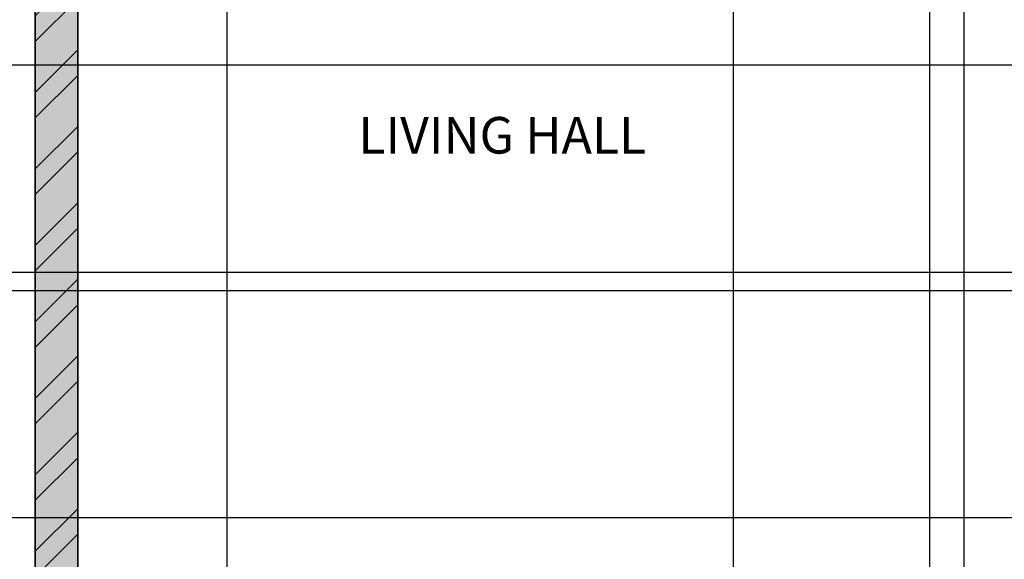
# Model space of a CAD drawing. Units: inches. Extents: x 1804 to 3296, y 909 to 2477.
# Tile 4 of 31: x 1922 to 2130, y 1215 to 1329. Entities that reach past the tile are written whole.
import ezdxf

# ---------------------------------------------------------------- set-up
doc = ezdxf.new("R2010")
doc.units = ezdxf.units.IN
for name, color, linetype, lineweight in [('A-ANNO-DIMS', 2, 'Continuous', 18), ('A-ANNO-TTLB', 156, 'Continuous', 35), ('A-AREA-IDEN', 190, 'Continuous', 18), ('A-WALL-PATT', 10, 'Continuous', 13), ('WALL', 10, 'Continuous', 35)]:
    doc.layers.add(name, color=color, linetype=linetype, lineweight=lineweight)
doc.styles.get("Standard").update_dxf_attribs({"font": 'arial.ttf'})
doc.dimstyles.new('ISO-25', dxfattribs={"dimtxt": 5, "dimasz": 2.5, "dimexe": 1.25, "dimexo": 0.625, "dimtad": 1, "dimdec": 0, "dimlunit": 4, "dimtxsty": 'Standard', "dimcen": 2.5, "dimadec": 0, "dimazin": 0, "dimtfac": 1, "dimtdec": 0, "dimtmove": 0, "dimatfit": 3, "dimfxl": 1, "dimarcsym": 0})

# ---------------------------------------------------------------- blocks, each defined once
blk = doc.blocks.new('*D21')
at = {"layer": 'A-ANNO-DIMS', "color": 0, "lineweight": -2, "transparency": 16777216}
for p, q in [((1935.21, 1539.88), (1967.44, 1539.88)), ((1966.19, 1149.57), (1966.19, 1537.38)), ((1935.21, 1147.07), (1967.44, 1147.07))]:
    blk.add_line(p, q, dxfattribs=at)
at = {"layer": 'A-ANNO-DIMS', "color": 0, "lineweight": 100, "transparency": 16777216}
for points in [[(1965.78, 1537.38), (1966.61, 1537.38), (1966.19, 1539.88)], [(1965.78, 1149.57), (1966.61, 1149.57), (1966.19, 1147.07)]]:
    blk.add_solid(points, dxfattribs=at)
at = {"layer": 'Defpoints', "color": 0, "lineweight": 100, "transparency": 16777216}
for p in [(1934.58, 1539.88), (1966.19, 1539.88), (1934.58, 1147.07)]:
    blk.add_point(p, dxfattribs=at)
at = {"layer": 'A-ANNO-DIMS', "color": 0, "transparency": 16777216, "insert": (1963.01, 1343.47), "char_height": 5, "attachment_point": 5, "rotation": 90}
blk.add_mtext('32\'-9"', dxfattribs=at)
blk = doc.blocks.new('*D52')
at = {"layer": 'A-ANNO-DIMS', "color": 0, "lineweight": -2, "transparency": 16777216}
for p, q in [((1924.96, 1830.04), (1880.63, 1830.04)), ((1881.88, 1065.27), (1881.88, 1827.54)), ((1924.96, 1062.77), (1880.63, 1062.77))]:
    blk.add_line(p, q, dxfattribs=at)
at = {"layer": 'A-ANNO-DIMS', "color": 0, "lineweight": 100, "transparency": 16777216}
for points in [[(1881.47, 1827.54), (1882.3, 1827.54), (1881.88, 1830.04)], [(1881.47, 1065.27), (1882.3, 1065.27), (1881.88, 1062.77)]]:
    blk.add_solid(points, dxfattribs=at)
at = {"layer": 'Defpoints', "color": 0, "lineweight": 100, "transparency": 16777216}
for p in [(1881.88, 1830.04), (1925.58, 1830.04), (1925.58, 1062.77)]:
    blk.add_point(p, dxfattribs=at)
at = {"layer": 'A-ANNO-DIMS', "color": 0, "transparency": 16777216, "insert": (1878.67, 1446.4), "char_height": 5, "attachment_point": 5, "rotation": 90}
blk.add_mtext('63\'-11 1/2"', dxfattribs=at)
blk = doc.blocks.new('*D59')
at = {"layer": 'A-ANNO-DIMS', "color": 0, "lineweight": -2, "transparency": 16777216}
for p, q in [((2121.83, 1590.3), (2121.83, 975.89)), ((2161.83, 1590.3), (2161.83, 975.89)), ((2124.33, 977.14), (2159.33, 977.14))]:
    blk.add_line(p, q, dxfattribs=at)
at = {"layer": 'A-ANNO-DIMS', "color": 0, "lineweight": 100, "transparency": 16777216}
for points in [[(2124.33, 977.56), (2124.33, 976.72), (2121.83, 977.14)], [(2159.33, 977.56), (2159.33, 976.72), (2161.83, 977.14)]]:
    blk.add_solid(points, dxfattribs=at)
at = {"layer": 'Defpoints', "color": 0, "lineweight": 100, "transparency": 16777216}
for p in [(2121.83, 1590.92), (2161.83, 1590.92), (2161.83, 977.14)]:
    blk.add_point(p, dxfattribs=at)
at = {"layer": 'A-ANNO-DIMS', "color": 0, "transparency": 16777216, "insert": (2141.83, 980.32), "char_height": 5, "attachment_point": 5}
blk.add_mtext('3\'-4"', dxfattribs=at)
blk = doc.blocks.new('*D60')
at = {"layer": 'A-ANNO-DIMS', "color": 0, "lineweight": -2, "transparency": 16777216}
for p, q in [((2073.08, 1544.95), (2073.08, 975.89)), ((2114.58, 1543.75), (2114.58, 975.89)), ((2112.08, 977.14), (2075.58, 977.14))]:
    blk.add_line(p, q, dxfattribs=at)
at = {"layer": 'A-ANNO-DIMS', "color": 0, "lineweight": 100, "transparency": 16777216}
for points in [[(2075.58, 977.56), (2075.58, 976.72), (2073.08, 977.14)], [(2112.08, 977.56), (2112.08, 976.72), (2114.58, 977.14)]]:
    blk.add_solid(points, dxfattribs=at)
at = {"layer": 'Defpoints', "color": 0, "lineweight": 100, "transparency": 16777216}
for p in [(2073.08, 1545.58), (2114.58, 1544.38), (2073.08, 977.14)]:
    blk.add_point(p, dxfattribs=at)
at = {"layer": 'A-ANNO-DIMS', "color": 0, "transparency": 16777216, "insert": (2093.83, 980.35), "char_height": 5, "attachment_point": 5}
blk.add_mtext('3\'-5 1/2"', dxfattribs=at)
blk = doc.blocks.new('*D63')
at = {"layer": 'A-ANNO-DIMS', "color": 0, "lineweight": -2, "transparency": 16777216}
for p, q in [((2157.95, 1319.33), (1880.63, 1319.33)), ((1881.88, 1277.99), (1881.88, 1316.83)), ((2157.95, 1275.49), (1880.63, 1275.49))]:
    blk.add_line(p, q, dxfattribs=at)
at = {"layer": 'A-ANNO-DIMS', "color": 0, "lineweight": 100, "transparency": 16777216}
for points in [[(1881.47, 1316.83), (1882.3, 1316.83), (1881.88, 1319.33)], [(1881.47, 1277.99), (1882.3, 1277.99), (1881.88, 1275.49)]]:
    blk.add_solid(points, dxfattribs=at)
at = {"layer": 'Defpoints', "color": 0, "lineweight": 100, "transparency": 16777216}
for p in [(1881.88, 1319.33), (2158.58, 1319.33), (2158.58, 1275.49)]:
    blk.add_point(p, dxfattribs=at)
at = {"layer": 'A-ANNO-DIMS', "color": 0, "transparency": 16777216, "insert": (1878.7, 1297.41), "char_height": 5, "attachment_point": 5, "rotation": 90}
blk.add_mtext('3\'-8"', dxfattribs=at)
blk = doc.blocks.new('*D70')
at = {"layer": 'A-ANNO-DIMS', "color": 0, "lineweight": -2, "transparency": 16777216}
for p, q in [((2208.56, 1271.63), (1880.63, 1271.63)), ((1881.88, 1226.13), (1881.88, 1269.13)), ((2208.56, 1223.63), (1880.63, 1223.63))]:
    blk.add_line(p, q, dxfattribs=at)
at = {"layer": 'A-ANNO-DIMS', "color": 0, "lineweight": 100, "transparency": 16777216}
for points in [[(1881.47, 1269.13), (1882.3, 1269.13), (1881.88, 1271.63)], [(1881.47, 1226.13), (1882.3, 1226.13), (1881.88, 1223.63)]]:
    blk.add_solid(points, dxfattribs=at)
at = {"layer": 'Defpoints', "color": 0, "lineweight": 100, "transparency": 16777216}
for p in [(1881.88, 1271.63), (2209.19, 1271.63), (2209.19, 1223.63)]:
    blk.add_point(p, dxfattribs=at)
at = {"layer": 'A-ANNO-DIMS', "color": 0, "transparency": 16777216, "insert": (1878.7, 1247.63), "char_height": 5, "attachment_point": 5, "rotation": 90}
blk.add_mtext('4\'-0"', dxfattribs=at)

msp = doc.modelspace()

# ---------------------------------------------------------------- hatches: boundary and pattern name
at = {"layer": 'A-ANNO-TTLB'}
h = msp.add_hatch(color=256, dxfattribs=at)
h.dxf.hatch_style = 1
h.paths.add_polyline_path([(3294.53, 2476.54), (1803.79, 2476.54), (1805.43, 909.47), (3296.17, 909.47)])
h.paths.add_polyline_path([(1811, 914.33), (1812.79, 2467.54), (3285.53, 2467.54), (3283.74, 914.33)], flags=16)
h.paths.add_polyline_path([(1925.58, 1062.77), (1925.58, 1138.07), (1925.58, 1539.88), (1925.58, 1793.38), (1925.58, 1830.04), (2325.54, 1830.04), (2325.54, 1793.38), (2325.54, 1586.42), (2325.54, 1138.07), (2325.54, 1062.77)], flags=0)
h.paths.add_polyline_path([(1997.22, 1029.4), (2008.85, 1037.96), (2008.85, 1020.84)], flags=0)
h.paths.add_polyline_path([(1934.58, 1138.07), (1934.58, 1147.07), (2078.77, 1147.07), (2078.77, 1138.07), (2060.94, 1138.07)], flags=0)
h.paths.add_polyline_path([(1944.35, 1138.07), (1944.35, 1147.07), (2056.05, 1147.07), (2056.05, 1138.07)], flags=0)
h.paths.add_polyline_path([(2222.24, 1037.96), (2233.87, 1029.4), (2222.24, 1020.84)], flags=0)
h.paths.add_polyline_path([(2061.94, 1139.07), (2061.94, 1146.07), (2077.77, 1146.07), (2077.77, 1139.07)], flags=0)
h.paths.add_polyline_path([(2149.58, 1138.07), (2149.58, 1269.44), (2158.58, 1269.44), (2158.58, 1326.69), (2149.58, 1326.69), (2149.58, 1340.94), (2139.6, 1340.94), (2139.6, 1434.25), (2149.58, 1434.25), (2149.58, 1447.36), (2158.58, 1447.36), (2158.58, 1423.87), (2158.58, 1408.06), (2198.46, 1408.06), (2198.46, 1412.56), (2282.65, 1412.56), (2282.65, 1465.94), (2316.54, 1465.94), (2316.54, 1590.92), (2192.86, 1590.92), (2192.86, 1595.3), (2291.17, 1595.3), (2291.17, 1590.92), (2316.54, 1590.92), (2316.54, 1784.38), (2300.24, 1784.38), (2300.24, 1757.47), (2268, 1757.47), (2268, 1681.04), (2180.87, 1681.04), (2180.87, 1757.47), (2148.63, 1757.47), (2148.63, 1784.38), (2119.08, 1784.38), (2119.08, 1585.58), (2114.58, 1585.58), (2114.58, 1784.38), (2064.11, 1784.38), (2046.28, 1784.38), (2046.28, 1760.38), (1958.58, 1760.38), (1958.58, 1664.38), (1934.58, 1664.38), (1934.58, 1784.38), (1934.58, 1793.38), (2046.28, 1793.38), (2064.11, 1793.38), (2119.08, 1793.38), (2230.78, 1793.38), (2230.78, 1784.38), (2268, 1784.38), (2300.24, 1784.38), (2316.54, 1784.38), (2316.54, 1590.92), (2316.54, 1373.73), (2316.54, 1138.07)], flags=0)
h.paths.add_polyline_path([(2209.19, 1166.63), (2209.19, 1175.63), (2158.58, 1175.63), (2209.19, 1223.63), (2209.19, 1231.63), (2183.88, 1231.63), (2183.88, 1301.66), (2242.59, 1301.66), (2242.59, 1326.69), (2316.54, 1326.69), (2272.59, 1271.63), (2272.59, 1223.63), (2316.54, 1175.63), (2272.59, 1175.63), (2272.59, 1166.63)], flags=0)
h.paths.add_polyline_path([(1947.77, 1345.22), (1947.77, 1457.48), (1991.2, 1457.48), (1991.2, 1451.7), (1991.2, 1352.18), (1991.2, 1345.22)], flags=0)
h.paths.add_polyline_path([(2209.19, 1271.63), (2262.59, 1271.63), (2262.59, 1311.85), (2272.59, 1301.66), (2272.59, 1271.63), (2269.92, 1269.63), (2270.59, 1269.63), (2270.59, 1225.63), (2211.19, 1225.63), (2211.19, 1269.63), (2211.86, 1269.63)], flags=0)
h.paths.add_polyline_path([(2000.34, 1378.21), (2000.34, 1429.71), (2025.22, 1429.71), (2025.22, 1378.21)], flags=0)
h.paths.add_polyline_path([(2001.34, 1379.21), (2001.34, 1428.71), (2024.22, 1428.71), (2024.22, 1379.21)], flags=0)
h.paths.add_polyline_path([(2012.34, 1390.21), (2012.34, 1417.71), (2013.22, 1417.71), (2013.22, 1390.21)], flags=0)
h.paths.add_polyline_path([(2237.56, 1331.19), (2237.56, 1340.18), (2238.62, 1340.18), (2238.62, 1386.84), (2241.04, 1386.84), (2242.06, 1386.84), (2242.06, 1408.06), (2316.54, 1331.19)], flags=0)
h.paths.add_polyline_path([(1953.73, 1464.35), (1953.73, 1498.59), (1981.74, 1498.59), (1981.74, 1464.35)], flags=0)
h.paths.add_polyline_path([(1987.63, 1462.08), (1987.63, 1500.95), (2104.07, 1500.95), (2104.07, 1462.08), (2099.27, 1462.08), (1993.6, 1462.08)], flags=0)
h.paths.add_polyline_path([(1956.06, 1481.47, -1), (1979.41, 1481.47, -1)], flags=0)
edge = h.paths.add_edge_path(flags=0)
edge.add_ellipse((2299.53, 1438.37), major_axis=(0.31, 21.36), ratio=0.670333, start_angle=0, end_angle=360)
h.paths.add_polyline_path([(2297.39, 1438.37, -1), (2301.67, 1438.37, -1)], flags=0)
h.paths.add_polyline_path([(2591.54, 1163.23), (2591.54, 1179.38), (2591.54, 1379.68), (2591.54, 1395.84), (2734.5, 1395.84), (2734.5, 1379.68), (2734.5, 1179.38), (2734.5, 1163.23)], flags=0)
h.paths.add_polyline_path([(2592.54, 1164.23), (2592.54, 1166.23), (2733.5, 1166.23), (2733.5, 1164.23)], flags=0)
h.paths.add_polyline_path([(2592.54, 1180.38), (2592.54, 1378.68), (2733.5, 1378.68), (2733.5, 1180.38)], flags=0)
h.paths.add_polyline_path([(2593.54, 1181.38), (2593.54, 1377.68), (2732.5, 1377.68), (2732.5, 1181.38)], flags=0)
h.paths.add_polyline_path([(2594.54, 1182.38), (2594.54, 1376.68), (2731.5, 1376.68), (2731.5, 1182.38)], flags=0)
h.paths.add_polyline_path([(1936.95, 1697.46), (1936.95, 1736.46), (1955.41, 1736.46), (1955.41, 1697.46)], flags=0)
h.paths.add_polyline_path([(1938.48, 1718.36), (1938.48, 1734.92), (1953.65, 1734.92), (1953.65, 1718.36)], flags=0)
h.paths.add_polyline_path([(1944.75, 1726.64, -1), (1947.37, 1726.64, -1)], flags=0)
h.paths.add_polyline_path([(2592.54, 1394.84), (2733.5, 1394.84), (2733.5, 1392.84), (2592.54, 1392.84)], flags=0)
h.paths.add_polyline_path([(1976.61, 1762.5), (1976.61, 1781.44), (2012.79, 1781.44), (2012.79, 1762.5)], flags=0)
h.paths.add_polyline_path([(1979.57, 1771.97, -1), (1991.39, 1771.97, -1)], flags=0)
h.paths.add_polyline_path([(1995.36, 1771.97, -1), (2007.18, 1771.97, -1)], flags=0)
h.paths.add_polyline_path([(2251.51, 1744.53), (2268, 1730.05), (2251.51, 1730.05)], flags=0)
h.paths.add_polyline_path([(2047.28, 1785.38), (2047.28, 1792.38), (2063.11, 1792.38), (2063.11, 1785.38)], flags=0)
h.paths.add_polyline_path([(2155.08, 1770.92, -1), (2174.42, 1770.92, -1)], flags=0)
h.paths.add_polyline_path([(2188.59, 1758.27), (2188.59, 1772.81), (2222.3, 1772.81), (2222.3, 1758.27)], flags=0)
h.paths.add_polyline_path([(2223.97, 1758.27), (2223.97, 1772.81), (2257.68, 1772.81), (2257.68, 1758.27)], flags=0)
h.paths.add_polyline_path([(2274.45, 1770.92, -1), (2293.8, 1770.92, -1)], flags=0)
h.paths.add_polyline_path([(2591.54, 1582.09), (2591.54, 1782.39), (2734.5, 1782.39), (2734.5, 1582.09)], flags=0)
h.paths.add_polyline_path([(2592.54, 1583.09), (2592.54, 1781.39), (2733.5, 1781.39), (2733.5, 1583.09)], flags=0)
h.paths.add_polyline_path([(2593.54, 1584.09), (2593.54, 1780.39), (2732.5, 1780.39), (2732.5, 1584.09)], flags=0)
h.paths.add_polyline_path([(2594.54, 1585.09), (2594.54, 1779.39), (2731.5, 1779.39), (2731.5, 1585.09)], flags=0)
h.paths.add_polyline_path([(1922.17, 1978.79), (1922.17, 2295.08), (1922.17, 2296.08), (2115.67, 2296.08), (2115.67, 2384.31), (2115.67, 2385.31), (2322.12, 2385.31), (2323.12, 2385.31), (2323.12, 1979.79), (2323.12, 1978.79), (1923.17, 1978.79)], flags=0)
h.paths.add_polyline_path([(1922.17, 1978.79), (1922.17, 2051.31), (1922.17, 2214.86), (1922.17, 2296.08), (2115.67, 2296.08), (2115.67, 2385.31), (2323.12, 2385.31), (2323.12, 2280.42), (2323.12, 1978.79), (2115.67, 1978.79)], flags=0)
h.paths.add_polyline_path([(1923.17, 1979.79), (1923.17, 2050.31), (2115.67, 2050.31), (2115.67, 2051.31), (1923.17, 2051.31), (1923.17, 2213.86), (1923.17, 2214.86), (1923.17, 2295.08), (1990.02, 2295.08), (1990.02, 2214.86), (1991.02, 2214.86), (1991.02, 2295.08), (2115.67, 2295.08), (2115.67, 1979.79), (2116.67, 1979.79), (2116.67, 2304.18), (2116.67, 2384.31), (2322.12, 2384.31), (2322.12, 2280.42), (2322.12, 1979.79), (2115.67, 1979.79)], flags=0)
h.paths.add_polyline_path([(2972.46, 1192.5), (2972.46, 1196.92), (2995.47, 1196.92), (2995.47, 1255.47), (2995.09, 1255.47), (2987.42, 1249.39), (2980.08, 1255.47), (2978.05, 1255.47), (2978.05, 1257.24), (2995.47, 1257.24), (2995.47, 1261.58), (3015.37, 1261.58), (3015.37, 1333.28), (3015.37, 1414.4), (3032.82, 1414.4), (3032.82, 1333.28), (3032.82, 1261.58), (3052.66, 1261.58), (3052.66, 1255.47), (3079.86, 1255.47), (3078.72, 1254.57), (3081.47, 1252.29), (3078.56, 1249.99), (3075.81, 1252.26), (3072.57, 1249.69), (3070.36, 1251.52), (3067.67, 1249.39), (3060.34, 1255.47), (3052.66, 1255.47), (3052.66, 1196.92), (3054.58, 1196.92), (3074, 1196.92), (3074, 1192.5), (3052.66, 1192.5), (2995.47, 1192.5)], flags=0)
h.paths.add_polyline_path([(2490.75, 1979.27), (2490.75, 1980.27), (2596.87, 1980.27), (2596.87, 2051.8), (2596.87, 2052.8), (2596.87, 2216.35), (2596.87, 2297.57), (2717.32, 2297.57), (2710.57, 2305.62), (2724.07, 2305.62), (2717.32, 2297.57), (2782.37, 2297.57), (2782.37, 2395.8), (3006.82, 2395.8), (3006.82, 1981.27), (3093.73, 1981.27), (3093.73, 1980.27), (3047.51, 1980.27), (3046.37, 1979.37), (3049.11, 1977.1), (3046.2, 1974.79), (3043.46, 1977.07), (3040.21, 1974.49), (3038, 1976.32), (3035.32, 1974.2), (3027.98, 1980.27), (2871.83, 1980.27), (2871.83, 1981.27), (2791.37, 1981.27), (2791.37, 2050.8), (2597.87, 2050.8), (2597.87, 1980.27), (2597.87, 1979.27), (2546.27, 1979.27), (2545.12, 1978.37), (2547.87, 1976.1), (2544.96, 1973.79), (2542.22, 1976.07), (2538.97, 1973.49), (2536.76, 1975.32), (2534.07, 1973.2), (2526.74, 1979.27)], flags=0)
h.paths.add_polyline_path([(2597.87, 2051.8), (2606.87, 2051.8), (2606.87, 2258.39), (2597.87, 2258.39), (2597.87, 2296.57), (2606.87, 2296.57), (2606.87, 2262.39), (2782.37, 2262.39), (2782.37, 2296.57), (2790.37, 2296.57), (2790.37, 2262.39), (2791.37, 2262.39), (2791.37, 2305.67), (2791.37, 2385.8), (2996.82, 2385.8), (2996.82, 2339.85), (3006.82, 2339.85), (3006.82, 2250.12), (2997.82, 2250.12), (2997.82, 1981.27), (2996.82, 1981.27), (2872.83, 1981.27), (2872.83, 1991.8), (2871.83, 1991.8), (2871.83, 2050.8), (2790.37, 2050.8), (2597.87, 2050.8)], flags=0)
h.paths.add_polyline_path([(2179.93, 2153.92), (2179.93, 2353.97), (2259.98, 2353.97), (2259.98, 2153.92)], flags=0)
h.paths.add_polyline_path([(2180.93, 2154.92), (2180.93, 2352.97), (2258.98, 2352.97), (2258.98, 2154.92)], flags=0)
h.paths.add_polyline_path([(2960.87, 1608.49), (2960.87, 1753.62), (3070.9, 1753.62), (3070.9, 1608.49)], flags=0)
h.paths.add_polyline_path([(2961.87, 1609.49), (2961.87, 1752.62), (3069.9, 1752.62), (3069.9, 1609.49)], flags=0)
h.paths.add_polyline_path([(2962.87, 1610.49), (2962.87, 1751.62), (3068.9, 1751.62), (3068.9, 1610.49)], flags=0)
h.paths.add_polyline_path([(2963.87, 1611.49), (2963.87, 1750.62), (3067.9, 1750.62), (3067.9, 1611.49)], flags=0)
h.paths.add_polyline_path([(2782.37, 2051.8), (2782.37, 2216.32), (2791.37, 2216.32), (2791.37, 2051.8), (2872.83, 2051.8), (2872.83, 2068.56), (2884.67, 2068.56), (2884.67, 2085.33), (2896.51, 2085.33), (2896.51, 2102.09), (2908.36, 2102.09), (2908.36, 2118.85), (2920.2, 2118.85), (2920.2, 2135.62), (2932.05, 2135.62), (2932.05, 2145.3), (2925.08, 2145.3), (2925.08, 2203.2), (2996.82, 2203.2), (2996.82, 2145.3), (2953.82, 2145.3), (2872.83, 2051.8), (2790.37, 2051.8)], flags=0)
h.paths.add_polyline_path([(2717.32, 2238.65), (2710.57, 2246.7), (2724.07, 2246.7)], flags=0)
h.paths.add_polyline_path([(2003.09, 1122.79), (2017.16, 1122.79), (2017.16, 1138.74), (2003.09, 1138.74)], flags=8)
h.paths.add_polyline_path([(2174.76, 1792.72), (2188.83, 1792.72), (2188.83, 1808.66), (2174.76, 1808.66)], flags=8)
h.paths.add_polyline_path([(1987.95, 1792.51), (2002.02, 1792.51), (2002.02, 1808.45), (1987.95, 1808.45)], flags=8)
h.paths.add_polyline_path([(2148.79, 1289.26), (2160.46, 1289.26), (2160.46, 1305.2), (2148.79, 1305.2)], flags=8)
h.paths.add_polyline_path([(2115.36, 1133.57), (2127.04, 1133.57), (2127.04, 1149.51), (2115.36, 1149.51)], flags=8)
h.paths.add_polyline_path([(2237.58, 1421.48), (2249.25, 1421.48), (2249.25, 1437.43), (2237.58, 1437.43)], flags=8)
h.paths.add_polyline_path([(2134.99, 1584.32), (2146.66, 1584.32), (2146.66, 1600.26), (2134.99, 1600.26)], flags=8)
h.paths.add_polyline_path([(2101.95, 1557.31), (2113.62, 1557.31), (2113.62, 1573.25), (2101.95, 1573.25)], flags=8)
h.paths.add_polyline_path([(2937.85, 1156.77), (3120.41, 1156.77), (3120.41, 1185.72), (2937.85, 1185.72)], flags=8)
h.paths.add_polyline_path([(2980.71, 1786.71), (3050.06, 1786.71), (3050.06, 1802.66), (2980.71, 1802.66)], flags=8)
h.paths.add_polyline_path([(2869.28, 1661.96), (2938.62, 1661.96), (2938.62, 1690.8), (2869.28, 1690.8)], flags=8)
h.paths.add_polyline_path([(3092.27, 1674.86), (3161.62, 1674.86), (3161.62, 1690.8), (3092.27, 1690.8)], flags=8)
h.paths.add_polyline_path([(2980.71, 1674.86), (3050.06, 1674.86), (3050.06, 1690.8), (2980.71, 1690.8)], flags=8)
h.paths.add_polyline_path([(2649.07, 1678.23), (2674.53, 1678.23), (2674.53, 1714.76), (2649.07, 1714.76)], flags=8)
h.paths.add_polyline_path([(2530.84, 1981.63), (2549.13, 1981.63), (2549.13, 1997.57), (2530.84, 1997.57)], flags=8)
h.paths.add_polyline_path([(3031.29, 1981.77), (3049.58, 1981.77), (3049.58, 1997.71), (3031.29, 1997.71)], flags=8)
h.paths.add_polyline_path([(2715.38, 1911.9), (2851.54, 1911.9), (2851.54, 1940.85), (2715.38, 1940.85)], flags=8)
h.paths.add_polyline_path([(2015.23, 1927.36), (2205.42, 1927.36), (2205.42, 1956.3), (2015.23, 1956.3)], flags=8)
h.paths.add_polyline_path([(2671.84, 2057.84), (2702.75, 2057.84), (2702.75, 2073.79), (2671.84, 2073.79)], flags=8)
h.paths.add_polyline_path([(2678.5, 2316.52), (2765.26, 2316.52), (2765.26, 2332.46), (2678.5, 2332.46)], flags=8)
h.paths.add_polyline_path([(2678.48, 2271.96), (2736.41, 2271.96), (2736.41, 2287.9), (2678.48, 2287.9)], flags=8)
h.paths.add_polyline_path([(2019.2, 972.79), (2243.21, 972.79), (2243.21, 1001.74), (2019.2, 1001.74)], flags=8)
h.paths.add_polyline_path([(2097.06, 1021.56), (2132.16, 1021.56), (2132.16, 1037.51), (2097.06, 1037.51)], flags=8)
h.paths.add_polyline_path([(2182.47, 1360.48), (2207.35, 1360.48), (2207.35, 1376.42), (2182.47, 1376.42)], flags=8)
h.paths.add_polyline_path([(2261.12, 1361.77), (2295.01, 1361.77), (2295.01, 1377.71), (2261.12, 1377.71)], flags=8)
h.paths.add_polyline_path([(2245.75, 1511.51), (2278.44, 1511.51), (2278.44, 1527.46), (2245.75, 1527.46)], flags=8)
h.paths.add_polyline_path([(1991.16, 1296.29), (2060.51, 1296.29), (2060.51, 1312.23), (1991.16, 1312.23)], flags=8)
h.paths.add_polyline_path([(2187, 1651.35), (2246.71, 1651.35), (2246.71, 1667.29), (2187, 1667.29)], flags=8)
h.paths.add_polyline_path([(1976.49, 1684.81), (2068.63, 1684.81), (2068.63, 1700.76), (1976.49, 1700.76)], flags=8)
at = {"layer": 'A-WALL-PATT'}
h = msp.add_hatch(color=256, dxfattribs=at)
h.dxf.hatch_style = 1
h.paths.add_polyline_path([(2119.08, 1544.38), (1925.58, 1544.38), (1925.58, 1539.88), (2119.08, 1539.88)])
h.paths.add_polyline_path([(2119.08, 1545.58), (2114.58, 1545.58), (2114.58, 1544.38), (2119.08, 1544.38)])
h.paths.add_polyline_path([(1965.87, 1658.79), (1965.87, 1679.09), (1955.57, 1679.09), (1955.57, 1658.79)], flags=9)
h.paths.add_polyline_path([(2293.18, 1677.29), (2293.18, 1697.58), (2282.88, 1697.58), (2282.88, 1677.29)], flags=9)
h.paths.add_polyline_path([(2271.13, 1545.23), (2287.53, 1545.23), (2287.53, 1555.53), (2271.13, 1555.53)], flags=9)
h.paths.add_polyline_path([(2303.26, 1488.52), (2303.26, 1508.82), (2292.95, 1508.82), (2292.95, 1488.52)], flags=9)
h.paths.add_polyline_path([(2271.13, 1393.15), (2287.53, 1393.15), (2287.53, 1403.45), (2271.13, 1403.45)], flags=9)
h.paths.add_polyline_path([(2306.48, 1361.45), (2306.48, 1377.86), (2296.18, 1377.86), (2296.18, 1361.45)], flags=9)
h.paths.add_polyline_path([(2174.54, 1361.45), (2174.54, 1377.86), (2164.23, 1377.86), (2164.23, 1361.45)], flags=9)
h.paths.add_polyline_path([(1968.21, 1333.34), (1968.21, 1353.64), (1957.91, 1353.64), (1957.91, 1333.34)], flags=9)
h.paths.add_polyline_path([(2003.09, 1122.79), (2017.16, 1122.79), (2017.16, 1138.74), (2003.09, 1138.74)], flags=9)
h.paths.add_polyline_path([(2174.76, 1792.72), (2188.83, 1792.72), (2188.83, 1808.66), (2174.76, 1808.66)], flags=9)
h.paths.add_polyline_path([(1987.95, 1792.51), (2002.02, 1792.51), (2002.02, 1808.45), (1987.95, 1808.45)], flags=9)
h.paths.add_polyline_path([(2148.79, 1289.26), (2160.46, 1289.26), (2160.46, 1305.2), (2148.79, 1305.2)], flags=9)
h.paths.add_polyline_path([(2115.36, 1133.57), (2127.04, 1133.57), (2127.04, 1149.51), (2115.36, 1149.51)], flags=9)
h.paths.add_polyline_path([(2237.58, 1421.48), (2249.25, 1421.48), (2249.25, 1437.43), (2237.58, 1437.43)], flags=9)
h.paths.add_polyline_path([(2134.99, 1584.32), (2146.66, 1584.32), (2146.66, 1600.26), (2134.99, 1600.26)], flags=9)
h.paths.add_polyline_path([(2101.95, 1557.31), (2113.62, 1557.31), (2113.62, 1573.25), (2101.95, 1573.25)], flags=9)
h.paths.add_polyline_path([(2937.85, 1156.77), (3120.41, 1156.77), (3120.41, 1185.72), (2937.85, 1185.72)], flags=9)
h.paths.add_polyline_path([(2980.71, 1786.71), (3050.06, 1786.71), (3050.06, 1802.66), (2980.71, 1802.66)], flags=9)
h.paths.add_polyline_path([(2869.28, 1661.96), (2938.62, 1661.96), (2938.62, 1690.8), (2869.28, 1690.8)], flags=9)
h.paths.add_polyline_path([(3092.27, 1674.86), (3161.62, 1674.86), (3161.62, 1690.8), (3092.27, 1690.8)], flags=9)
h.paths.add_polyline_path([(2980.71, 1674.86), (3050.06, 1674.86), (3050.06, 1690.8), (2980.71, 1690.8)], flags=9)
h.paths.add_polyline_path([(2649.07, 1678.23), (2674.53, 1678.23), (2674.53, 1714.76), (2649.07, 1714.76)], flags=9)
h.paths.add_polyline_path([(2530.84, 1981.63), (2549.13, 1981.63), (2549.13, 1997.57), (2530.84, 1997.57)], flags=9)
h.paths.add_polyline_path([(3031.29, 1981.77), (3049.58, 1981.77), (3049.58, 1997.71), (3031.29, 1997.71)], flags=9)
h.paths.add_polyline_path([(2715.38, 1911.9), (2851.54, 1911.9), (2851.54, 1940.85), (2715.38, 1940.85)], flags=9)
h.paths.add_polyline_path([(2015.23, 1927.36), (2205.42, 1927.36), (2205.42, 1956.3), (2015.23, 1956.3)], flags=9)
h.paths.add_polyline_path([(2671.84, 2057.84), (2702.75, 2057.84), (2702.75, 2073.79), (2671.84, 2073.79)], flags=9)
h.paths.add_polyline_path([(2678.5, 2316.52), (2765.26, 2316.52), (2765.26, 2332.46), (2678.5, 2332.46)], flags=9)
h.paths.add_polyline_path([(2678.48, 2271.96), (2736.41, 2271.96), (2736.41, 2287.9), (2678.48, 2287.9)], flags=9)
h.paths.add_polyline_path([(2019.2, 972.79), (2243.21, 972.79), (2243.21, 1001.74), (2019.2, 1001.74)], flags=9)
h.paths.add_polyline_path([(2097.06, 1021.56), (2132.16, 1021.56), (2132.16, 1037.51), (2097.06, 1037.51)], flags=9)
h.paths.add_polyline_path([(2182.47, 1360.48), (2207.35, 1360.48), (2207.35, 1376.42), (2182.47, 1376.42)], flags=9)
h.paths.add_polyline_path([(2261.12, 1361.77), (2295.01, 1361.77), (2295.01, 1377.71), (2261.12, 1377.71)], flags=9)
h.paths.add_polyline_path([(2245.75, 1511.51), (2278.44, 1511.51), (2278.44, 1527.46), (2245.75, 1527.46)], flags=9)
h.paths.add_polyline_path([(1991.16, 1296.29), (2060.51, 1296.29), (2060.51, 1312.23), (1991.16, 1312.23)], flags=9)
h.paths.add_polyline_path([(2187, 1651.35), (2246.71, 1651.35), (2246.71, 1667.29), (2187, 1667.29)], flags=9)
h.paths.add_polyline_path([(1976.49, 1684.81), (2068.63, 1684.81), (2068.63, 1700.76), (1976.49, 1700.76)], flags=9)
h = msp.add_hatch(color=256, dxfattribs=at)
h.dxf.hatch_style = 1
h.paths.add_polyline_path([(2149.58, 1147.07), (2141.21, 1147.07), (2141.21, 1144.07), (2141.21, 1138.07), (2149.58, 1138.07)])
h.paths.add_polyline_path([(2101.21, 1144.07, -0.01877), (2101.32, 1147.07), (2078.77, 1147.07), (2078.77, 1138.07), (2101.21, 1138.07)])
h.paths.add_polyline_path([(2060.94, 1147.07), (2056.05, 1147.07), (2056.05, 1138.07), (2060.94, 1138.07)])
h.paths.add_polyline_path([(1944.35, 1147.07), (1934.58, 1147.07), (1934.58, 1138.07), (1944.35, 1138.07)])
h.paths.add_polyline_path([(2158.58, 1269.44), (2149.58, 1269.44), (2149.58, 1138.07), (2158.58, 1138.07)])
h.paths.add_polyline_path([(2003.09, 1122.79), (2017.16, 1122.79), (2017.16, 1138.74), (2003.09, 1138.74)], flags=9)
h.paths.add_polyline_path([(2174.76, 1792.72), (2188.83, 1792.72), (2188.83, 1808.66), (2174.76, 1808.66)], flags=9)
h.paths.add_polyline_path([(1987.95, 1792.51), (2002.02, 1792.51), (2002.02, 1808.45), (1987.95, 1808.45)], flags=9)
h.paths.add_polyline_path([(2148.79, 1289.26), (2160.46, 1289.26), (2160.46, 1305.2), (2148.79, 1305.2)], flags=9)
h.paths.add_polyline_path([(2115.36, 1133.57), (2127.04, 1133.57), (2127.04, 1149.51), (2115.36, 1149.51)], flags=9)
h.paths.add_polyline_path([(2237.58, 1421.48), (2249.25, 1421.48), (2249.25, 1437.43), (2237.58, 1437.43)], flags=9)
h.paths.add_polyline_path([(2134.99, 1584.32), (2146.66, 1584.32), (2146.66, 1600.26), (2134.99, 1600.26)], flags=9)
h.paths.add_polyline_path([(2101.95, 1557.31), (2113.62, 1557.31), (2113.62, 1573.25), (2101.95, 1573.25)], flags=9)
h.paths.add_polyline_path([(2937.85, 1156.77), (3120.41, 1156.77), (3120.41, 1185.72), (2937.85, 1185.72)], flags=9)
h.paths.add_polyline_path([(2980.71, 1786.71), (3050.06, 1786.71), (3050.06, 1802.66), (2980.71, 1802.66)], flags=9)
h.paths.add_polyline_path([(2869.28, 1661.96), (2938.62, 1661.96), (2938.62, 1690.8), (2869.28, 1690.8)], flags=9)
h.paths.add_polyline_path([(3092.27, 1674.86), (3161.62, 1674.86), (3161.62, 1690.8), (3092.27, 1690.8)], flags=9)
h.paths.add_polyline_path([(2980.71, 1674.86), (3050.06, 1674.86), (3050.06, 1690.8), (2980.71, 1690.8)], flags=9)
h.paths.add_polyline_path([(2649.07, 1678.23), (2674.53, 1678.23), (2674.53, 1714.76), (2649.07, 1714.76)], flags=9)
h.paths.add_polyline_path([(2530.84, 1981.63), (2549.13, 1981.63), (2549.13, 1997.57), (2530.84, 1997.57)], flags=9)
h.paths.add_polyline_path([(3031.29, 1981.77), (3049.58, 1981.77), (3049.58, 1997.71), (3031.29, 1997.71)], flags=9)
h.paths.add_polyline_path([(2715.38, 1911.9), (2851.54, 1911.9), (2851.54, 1940.85), (2715.38, 1940.85)], flags=9)
h.paths.add_polyline_path([(2015.23, 1927.36), (2205.42, 1927.36), (2205.42, 1956.3), (2015.23, 1956.3)], flags=9)
h.paths.add_polyline_path([(2671.84, 2057.84), (2702.75, 2057.84), (2702.75, 2073.79), (2671.84, 2073.79)], flags=9)
h.paths.add_polyline_path([(2678.5, 2316.52), (2765.26, 2316.52), (2765.26, 2332.46), (2678.5, 2332.46)], flags=9)
h.paths.add_polyline_path([(2678.48, 2271.96), (2736.41, 2271.96), (2736.41, 2287.9), (2678.48, 2287.9)], flags=9)
h.paths.add_polyline_path([(2019.2, 972.79), (2243.21, 972.79), (2243.21, 1001.74), (2019.2, 1001.74)], flags=9)
h.paths.add_polyline_path([(2097.06, 1021.56), (2132.16, 1021.56), (2132.16, 1037.51), (2097.06, 1037.51)], flags=9)
h.paths.add_polyline_path([(2182.47, 1360.48), (2207.35, 1360.48), (2207.35, 1376.42), (2182.47, 1376.42)], flags=9)
h.paths.add_polyline_path([(2261.12, 1361.77), (2295.01, 1361.77), (2295.01, 1377.71), (2261.12, 1377.71)], flags=9)
h.paths.add_polyline_path([(2245.75, 1511.51), (2278.44, 1511.51), (2278.44, 1527.46), (2245.75, 1527.46)], flags=9)
h.paths.add_polyline_path([(1991.16, 1296.29), (2060.51, 1296.29), (2060.51, 1312.23), (1991.16, 1312.23)], flags=9)
h.paths.add_polyline_path([(2187, 1651.35), (2246.71, 1651.35), (2246.71, 1667.29), (2187, 1667.29)], flags=9)
h.paths.add_polyline_path([(1976.49, 1684.81), (2068.63, 1684.81), (2068.63, 1700.76), (1976.49, 1700.76)], flags=9)
h = msp.add_hatch(color=256, dxfattribs=at)
h.dxf.hatch_style = 1
h.paths.add_polyline_path([(2158.58, 1275.49), (2155.29, 1275.49), (2149.58, 1275.49), (2149.58, 1269.44), (2158.58, 1269.44)])
h.paths.add_polyline_path([(2158.58, 1326.69), (2149.58, 1326.69), (2149.58, 1319.33), (2155.29, 1319.33), (2158.58, 1319.33)])
h.paths.add_polyline_path([(2158.58, 1402.2), (2158.58, 1423.87), (2158.58, 1447.36), (2149.58, 1447.36), (2149.58, 1423.87), (2149.58, 1340.94), (2149.58, 1326.69), (2158.58, 1326.69), (2158.58, 1354.23)])
h.paths.add_polyline_path([(1965.87, 1658.79), (1965.87, 1679.09), (1955.57, 1679.09), (1955.57, 1658.79)], flags=9)
h.paths.add_polyline_path([(2293.18, 1677.29), (2293.18, 1697.58), (2282.88, 1697.58), (2282.88, 1677.29)], flags=9)
h.paths.add_polyline_path([(2271.13, 1545.23), (2287.53, 1545.23), (2287.53, 1555.53), (2271.13, 1555.53)], flags=9)
h.paths.add_polyline_path([(2303.26, 1488.52), (2303.26, 1508.82), (2292.95, 1508.82), (2292.95, 1488.52)], flags=9)
h.paths.add_polyline_path([(2271.13, 1393.15), (2287.53, 1393.15), (2287.53, 1403.45), (2271.13, 1403.45)], flags=9)
h.paths.add_polyline_path([(2306.48, 1361.45), (2306.48, 1377.86), (2296.18, 1377.86), (2296.18, 1361.45)], flags=9)
h.paths.add_polyline_path([(2189.9, 1340.62), (2206.31, 1340.62), (2206.31, 1350.92), (2189.9, 1350.92)], flags=9)
h.paths.add_polyline_path([(2174.54, 1361.45), (2174.54, 1377.86), (2164.23, 1377.86), (2164.23, 1361.45)], flags=9)
h.paths.add_polyline_path([(2304.24, 1240.8), (2304.24, 1261.09), (2293.94, 1261.09), (2293.94, 1240.8)], flags=9)
h.paths.add_polyline_path([(2227.19, 1188.73), (2247.49, 1188.73), (2247.49, 1199.03), (2227.19, 1199.03)], flags=9)
h.paths.add_polyline_path([(2181.93, 1144.21), (2181.93, 1160.62), (2171.63, 1160.62), (2171.63, 1144.21)], flags=9)
h.paths.add_polyline_path([(1968.21, 1333.34), (1968.21, 1353.64), (1957.91, 1353.64), (1957.91, 1333.34)], flags=9)
h.paths.add_polyline_path([(2029.78, 1203.53), (2053.95, 1203.53), (2053.95, 1213.83), (2029.78, 1213.83)], flags=9)
h.paths.add_polyline_path([(2576.51, 1671.88), (2576.51, 1692.17), (2566.21, 1692.17), (2566.21, 1671.88)], flags=9)
h.paths.add_polyline_path([(2566.99, 1269.67), (2566.99, 1289.96), (2556.68, 1289.96), (2556.68, 1269.67)], flags=9)
h.paths.add_polyline_path([(2581.85, 1269.17), (2581.85, 1289.46), (2571.54, 1289.46), (2571.54, 1269.17)], flags=9)
h.paths.add_polyline_path([(2650.71, 1409.75), (2674.89, 1409.75), (2674.89, 1420.05), (2650.71, 1420.05)], flags=9)
h.paths.add_polyline_path([(2003.09, 1122.79), (2017.16, 1122.79), (2017.16, 1138.74), (2003.09, 1138.74)], flags=9)
h.paths.add_polyline_path([(2174.76, 1792.72), (2188.83, 1792.72), (2188.83, 1808.66), (2174.76, 1808.66)], flags=9)
h.paths.add_polyline_path([(1987.95, 1792.51), (2002.02, 1792.51), (2002.02, 1808.45), (1987.95, 1808.45)], flags=9)
h.paths.add_polyline_path([(2148.79, 1289.26), (2160.46, 1289.26), (2160.46, 1305.2), (2148.79, 1305.2)], flags=9)
h.paths.add_polyline_path([(2115.36, 1133.57), (2127.04, 1133.57), (2127.04, 1149.51), (2115.36, 1149.51)], flags=9)
h.paths.add_polyline_path([(2237.58, 1421.48), (2249.25, 1421.48), (2249.25, 1437.43), (2237.58, 1437.43)], flags=9)
h.paths.add_polyline_path([(2134.99, 1584.32), (2146.66, 1584.32), (2146.66, 1600.26), (2134.99, 1600.26)], flags=9)
h.paths.add_polyline_path([(2101.95, 1557.31), (2113.62, 1557.31), (2113.62, 1573.25), (2101.95, 1573.25)], flags=9)
h.paths.add_polyline_path([(2937.85, 1156.77), (3120.41, 1156.77), (3120.41, 1185.72), (2937.85, 1185.72)], flags=9)
h.paths.add_polyline_path([(2980.71, 1786.71), (3050.06, 1786.71), (3050.06, 1802.66), (2980.71, 1802.66)], flags=9)
h.paths.add_polyline_path([(2869.28, 1661.96), (2938.62, 1661.96), (2938.62, 1690.8), (2869.28, 1690.8)], flags=9)
h.paths.add_polyline_path([(3092.27, 1674.86), (3161.62, 1674.86), (3161.62, 1690.8), (3092.27, 1690.8)], flags=9)
h.paths.add_polyline_path([(2980.71, 1674.86), (3050.06, 1674.86), (3050.06, 1690.8), (2980.71, 1690.8)], flags=9)
h.paths.add_polyline_path([(2649.07, 1678.23), (2674.53, 1678.23), (2674.53, 1714.76), (2649.07, 1714.76)], flags=9)
h.paths.add_polyline_path([(2530.84, 1981.63), (2549.13, 1981.63), (2549.13, 1997.57), (2530.84, 1997.57)], flags=9)
h.paths.add_polyline_path([(3031.29, 1981.77), (3049.58, 1981.77), (3049.58, 1997.71), (3031.29, 1997.71)], flags=9)
h.paths.add_polyline_path([(2715.38, 1911.9), (2851.54, 1911.9), (2851.54, 1940.85), (2715.38, 1940.85)], flags=9)
h.paths.add_polyline_path([(2015.23, 1927.36), (2205.42, 1927.36), (2205.42, 1956.3), (2015.23, 1956.3)], flags=9)
h.paths.add_polyline_path([(2671.84, 2057.84), (2702.75, 2057.84), (2702.75, 2073.79), (2671.84, 2073.79)], flags=9)
h.paths.add_polyline_path([(2678.5, 2316.52), (2765.26, 2316.52), (2765.26, 2332.46), (2678.5, 2332.46)], flags=9)
h.paths.add_polyline_path([(2678.48, 2271.96), (2736.41, 2271.96), (2736.41, 2287.9), (2678.48, 2287.9)], flags=9)
h.paths.add_polyline_path([(2019.2, 972.79), (2243.21, 972.79), (2243.21, 1001.74), (2019.2, 1001.74)], flags=9)
h.paths.add_polyline_path([(2097.06, 1021.56), (2132.16, 1021.56), (2132.16, 1037.51), (2097.06, 1037.51)], flags=9)
h.paths.add_polyline_path([(2182.47, 1360.48), (2207.35, 1360.48), (2207.35, 1376.42), (2182.47, 1376.42)], flags=9)
h.paths.add_polyline_path([(2261.12, 1361.77), (2295.01, 1361.77), (2295.01, 1377.71), (2261.12, 1377.71)], flags=9)
h.paths.add_polyline_path([(2245.75, 1511.51), (2278.44, 1511.51), (2278.44, 1527.46), (2245.75, 1527.46)], flags=9)
h.paths.add_polyline_path([(1991.16, 1296.29), (2060.51, 1296.29), (2060.51, 1312.23), (1991.16, 1312.23)], flags=9)
h.paths.add_polyline_path([(2187, 1651.35), (2246.71, 1651.35), (2246.71, 1667.29), (2187, 1667.29)], flags=9)
h.paths.add_polyline_path([(1976.49, 1684.81), (2068.63, 1684.81), (2068.63, 1700.76), (1976.49, 1700.76)], flags=9)
h = msp.add_hatch(dxfattribs=at)
h.set_pattern_fill('ANSI32', color=256, scale=1.2)
h.set_pattern_definition([(45, (0, 196.207), (-8.08223, 8.08223), []), (45, (5.388, 196.207), (-8.08223, 8.08223), [])])
h.paths.add_polyline_path([(1934.58, 1784.38), (1934.58, 1793.38), (1925.58, 1793.38), (1925.58, 1539.88), (2119.08, 1539.88), (2119.08, 1545.58), (2114.58, 1545.58), (2114.58, 1544.38), (1934.58, 1544.38)])
h.paths.add_polyline_path([(2114.58, 1793.38), (2064.11, 1793.38), (2064.11, 1784.38), (2114.58, 1784.38)], flags=17)
h.paths.add_polyline_path([(2325.54, 1793.38), (2230.78, 1793.38), (2230.78, 1784.38), (2268, 1784.38), (2300.24, 1784.38), (2316.54, 1784.38), (2316.54, 1590.92), (2316.54, 1586.42), (2325.54, 1586.42)])
h.paths.add_polyline_path([(1944.35, 1147.07), (1934.58, 1147.07), (1934.58, 1138.07), (1944.35, 1138.07)])
h.paths.add_polyline_path([(2101.21, 1144.07, -0.01877), (2101.32, 1147.07), (2078.77, 1147.07), (2078.77, 1138.07), (2101.21, 1138.07)])
h.paths.add_polyline_path([(1934.58, 1539.88), (1925.58, 1539.88), (1925.58, 1138.07), (1934.58, 1138.07), (1934.58, 1147.07)])
h.paths.add_polyline_path([(2325.54, 1586.42), (2316.54, 1586.42), (2316.54, 1373.73), (2316.54, 1138.07), (2325.54, 1138.07), (2325.54, 1228.97)])
h.paths.add_polyline_path([(2158.58, 1423.87), (2158.58, 1447.36), (2149.58, 1447.36), (2149.58, 1423.87), (2149.58, 1340.94), (2149.58, 1326.69), (2158.58, 1326.69), (2158.58, 1354.23), (2158.58, 1402.2)])
h.paths.add_polyline_path([(2316.54, 1412.56), (2282.65, 1412.56), (2273.09, 1412.56), (2273.09, 1408.06), (2316.54, 1408.06)])
h.paths.add_polyline_path([(2273.09, 1412.56), (2242.06, 1412.56), (2242.06, 1408.06), (2273.09, 1408.06)])
h.paths.add_polyline_path([(2237.56, 1412.56), (2198.46, 1412.56), (2198.46, 1408.06), (2237.56, 1408.06)])
h.paths.add_polyline_path([(2242.06, 1408.06), (2237.56, 1408.06), (2237.56, 1386.84), (2242.06, 1386.84)])
h.paths.add_polyline_path([(2242.06, 1412.56), (2237.56, 1412.56), (2237.56, 1408.06), (2242.06, 1408.06)])
h.paths.add_polyline_path([(2158.58, 1269.44), (2149.58, 1269.44), (2149.58, 1138.07), (2158.58, 1138.07)])
h.paths.add_polyline_path([(2149.58, 1147.07), (2141.21, 1147.07), (2141.21, 1144.07), (2141.21, 1138.07), (2149.58, 1138.07)])
h.paths.add_polyline_path([(2272.59, 1175.63), (2209.19, 1175.63), (2209.19, 1166.63), (2272.59, 1166.63)])
h.paths.add_polyline_path([(2237.56, 1446.21), (2242.06, 1446.21), (2242.06, 1586.42), (2237.56, 1586.42)])
h.paths.add_polyline_path([(2242.06, 1414.58), (2237.56, 1414.58), (2237.56, 1412.56), (2242.06, 1412.56)])
h = msp.add_hatch(color=256, dxfattribs=at)
h.dxf.hatch_style = 1
h.paths.add_polyline_path([(1934.58, 1793.38), (1925.58, 1793.38), (1925.58, 1544.38), (1934.58, 1544.38)])
h.paths.add_polyline_path([(1934.58, 1539.88), (1925.58, 1539.88), (1925.58, 1138.07), (1934.58, 1138.07)])

# ---------------------------------------------------------------- linework, layer by layer
at = {"layer": 'WALL'}
for p, q in [((1925.58, 1539.88), (1925.58, 1138.07)), ((1934.58, 1539.88), (1934.58, 1138.07))]:
    msp.add_line(p, q, dxfattribs=at)
msp.add_lwpolyline([(1925.58, 1138.07), (1934.58, 1138.07), (1934.58, 1539.88), (1925.58, 1539.88)], close=True, dxfattribs=at)

# ---------------------------------------------------------------- texts
at = {"layer": 'A-AREA-IDEN', "insert": (1993.89, 1308.38), "char_height": 7.7373, "attachment_point": 1}
msp.add_mtext_dynamic_manual_height_columns('LIVING HALL', width=163.3261, gutter_width=38.69, heights=[0], dxfattribs=at)

# ---------------------------------------------------------------- dimensions: what is measured, and where the dimension line sits
at = {"layer": 'A-ANNO-DIMS'}
for base, p1, p2, override, picture, middle in [((1881.88, 1830.04), (1925.58, 1062.77), (1925.58, 1830.04), {"dimdec": 1, "dimlfac": 1, "dimrnd": 0, "dimzin": 1, "dimdsep": 46, "dimlunit": 4, "dimfrac": 2}, '*D52', (1878.67, 1446.4)), ((1966.19, 1539.88), (1934.58, 1147.07), (1934.58, 1539.88), {"dimclrd": 0, "dimclre": 0, "dimclrt": 0}, '*D21', (1963.01, 1343.47)), ((1881.88, 1319.33), (2158.58, 1275.49), (2158.58, 1319.33), {"dimdec": 1, "dimlfac": 1, "dimrnd": 0, "dimzin": 1, "dimdsep": 46, "dimlunit": 4, "dimfrac": 2}, '*D63', (1878.7, 1297.41)), ((1881.88, 1271.63), (2209.19, 1223.63), (2209.19, 1271.63), {"dimdec": 1, "dimlfac": 1, "dimrnd": 0, "dimzin": 1, "dimdsep": 46, "dimlunit": 4, "dimfrac": 2}, '*D70', (1878.7, 1247.63))]:
    dim = msp.add_linear_dim(base=base, p1=p1, p2=p2, angle=90, dimstyle='ISO-25', override=override, dxfattribs=at)
    dim.commit()
    dim.dimension.update_dxf_attribs({"geometry": picture, "text_midpoint": middle})
for base, p1, p2, picture, middle in [((2161.83, 977.14), (2121.83, 1590.92), (2161.83, 1590.92), '*D59', (2141.83, 980.32)), ((2073.08, 977.14), (2114.58, 1544.38), (2073.08, 1545.58), '*D60', (2093.83, 980.35))]:
    dim = msp.add_linear_dim(base=base, p1=p1, p2=p2, dimstyle='ISO-25', override={"dimdec": 1, "dimlfac": 1, "dimrnd": 0, "dimzin": 1, "dimdsep": 46, "dimlunit": 4, "dimfrac": 2}, dxfattribs=at)
    dim.commit()
    dim.dimension.update_dxf_attribs({"geometry": picture, "text_midpoint": middle})

doc.saveas('drawing.dxf')
